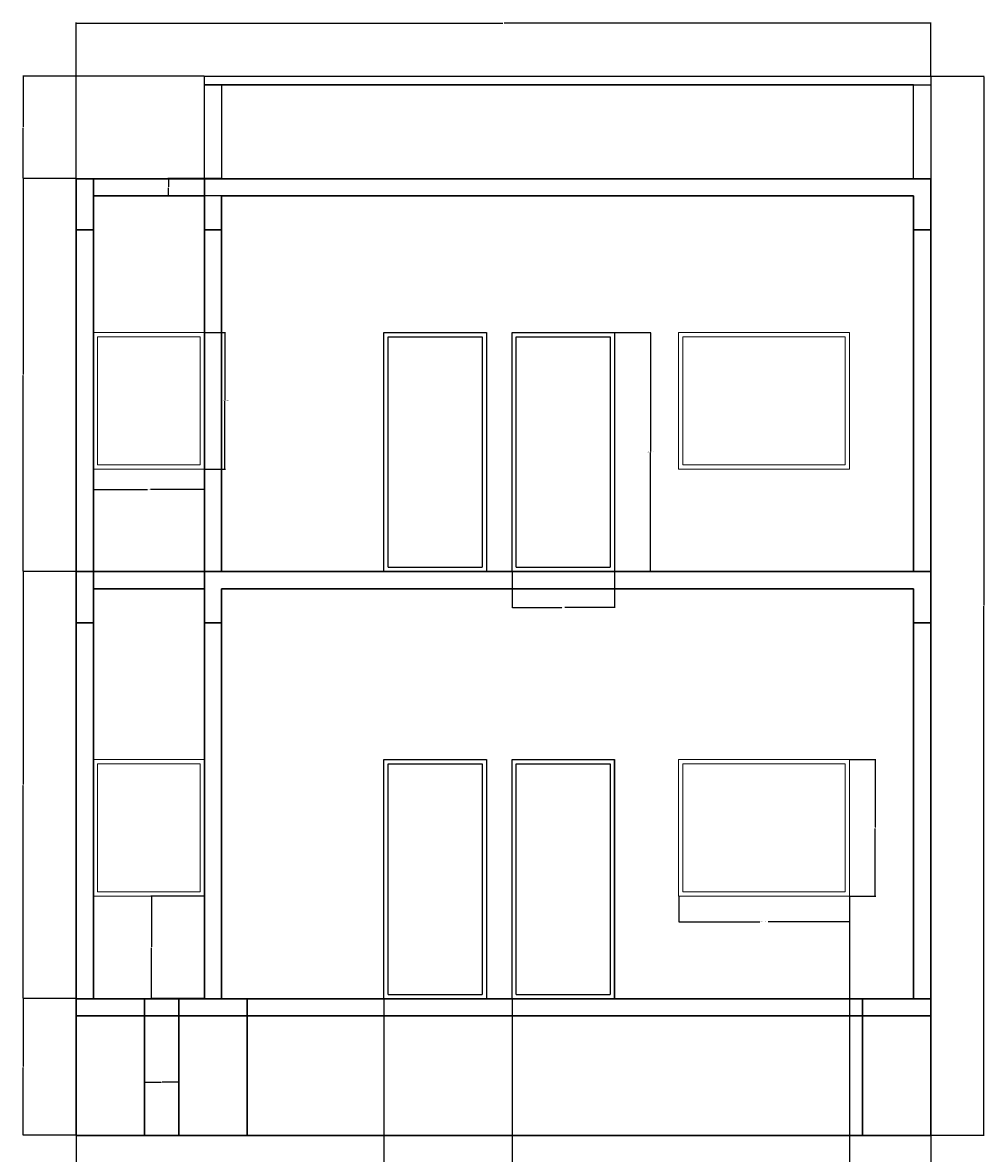
# Model space of a CAD drawing. Units: millimetres. Extents: x 1831 to 2754, y 1517 to 2450.
# Tile 4 of 4: x 2413 to 2751, y 1965 to 2362. Entities that reach past the tile are written whole.
import ezdxf

# ---------------------------------------------------------------- set-up
doc = ezdxf.new("R2010")
doc.units = ezdxf.units.MM
for name, color, linetype, lineweight in [('A-ANNO-DIMS', 2, 'Continuous', 18), ('A-DOOR', 3, 'Continuous', 25), ('A-ELEV-BASE', 7, 'Continuous', 30), ('A-GLAZ', 4, 'Continuous', 18), ('A-ROOF', 7, 'Continuous', 25), ('A-SECT', 7, 'Continuous', 30)]:
    doc.layers.add(name, color=color, linetype=linetype, lineweight=lineweight)
doc.styles.get("Standard").update_dxf_attribs({"font": 'arial.ttf'})
doc.dimstyles.get("Standard").update_dxf_attribs({"dimtxt": 0.18, "dimasz": 0.18, "dimexe": 0.18, "dimexo": 0.0625, "dimgap": 0.09, "dimtad": 0, "dimtih": 1, "dimtoh": 1, "dimdec": 4, "dimzin": 0, "dimdsep": 46, "dimtxsty": 'Standard', "dimcen": 0.09, "dimadec": 0, "dimazin": 0, "dimtfac": 1, "dimtdec": 4, "dimtofl": 0, "dimtmove": 0, "dimatfit": 3, "dimfxl": 1, "dimtolj": 1, "dimtzin": 0, "dimarcsym": 0})

# ---------------------------------------------------------------- blocks, each defined once
blk = doc.blocks.new('DOOR-SECT-FRAMED')
for p, q in [((0, 0), (0, 84)), ((0, 84), (36, 84)), ((36, 84), (36, 0)), ((1.5, 82.5), (34.5, 82.5)), ((1.5, 1.5), (1.5, 82.5)), ((34.5, 82.5), (34.5, 1.5)), ((1.5, 1.5), (34.5, 1.5))]:
    blk.add_line(p, q)
blk = doc.blocks.new('WINDOW-SECT-WIDE')
for p, q in [((0, 48), (60, 48)), ((30, 48), (0, 48)), ((0, 48), (0, 0)), ((60, 48), (30, 48)), ((60, 0), (60, 48)), ((30, 46.5), (1.5, 46.5)), ((1.5, 46.5), (1.5, 1.5)), ((58.5, 46.5), (30, 46.5)), ((58.5, 1.5), (58.5, 46.5)), ((1.5, 1.5), (58.5, 1.5)), ((0, 0), (60, 0))]:
    blk.add_line(p, q)
blk = doc.blocks.new('WINDOW-SECT-NARROW')
for p, q in [((0, 48), (39, 48)), ((39, 48), (39, 0)), ((1.5, 46.5), (37.5, 46.5)), ((1.5, 1.5), (1.5, 46.5)), ((37.5, 46.5), (37.5, 1.5)), ((37.5, 1.5), (1.5, 1.5)), ((39, 0), (0, 0))]:
    blk.add_line(p, q)
blk = doc.blocks.new('*D8')
at = {"layer": 'A-ANNO-DIMS', "color": 0, "lineweight": -2, "transparency": 16777216}
for p, q in [((2620.82, 2253.57), (2633.54, 2253.57)), ((2633.36, 2253.39), (2633.36, 2211.75)), ((2633.36, 2169.75), (2633.36, 2211.38)), ((2620.82, 2169.57), (2633.54, 2169.57))]:
    blk.add_line(p, q, dxfattribs=at)
at = {"layer": 'A-ANNO-DIMS', "color": 0, "transparency": 16777216}
for points in [[(2633.33, 2253.39), (2633.39, 2253.39), (2633.36, 2253.57)], [(2633.33, 2169.75), (2633.39, 2169.75), (2633.36, 2169.57)]]:
    blk.add_solid(points, dxfattribs=at)
at = {"layer": 'Defpoints', "color": 0, "transparency": 16777216}
for p in [(2620.76, 2253.57), (2633.36, 2253.57), (2620.76, 2169.57)]:
    blk.add_point(p, dxfattribs=at)
at = {"layer": 'A-ANNO-DIMS', "color": 0, "transparency": 16777216, "insert": (2633.36, 2211.57), "char_height": 0.18, "attachment_point": 5}
blk.add_mtext('\\A1;FRAMED DOOR 84 TYP.', dxfattribs=at)
blk = doc.blocks.new('*D9')
at = {"layer": 'A-ANNO-DIMS', "color": 0, "lineweight": -2, "transparency": 16777216}
for p, q in [((2584.76, 2169.5), (2584.76, 2156.79)), ((2620.76, 2169.5), (2620.76, 2156.79)), ((2584.94, 2156.97), (2602.23, 2156.97)), ((2620.58, 2156.97), (2603.29, 2156.97))]:
    blk.add_line(p, q, dxfattribs=at)
at = {"layer": 'A-ANNO-DIMS', "color": 0, "transparency": 16777216}
for points in [[(2584.94, 2157), (2584.94, 2156.94), (2584.76, 2156.97)], [(2620.58, 2157), (2620.58, 2156.94), (2620.76, 2156.97)]]:
    blk.add_solid(points, dxfattribs=at)
at = {"layer": 'Defpoints', "color": 0, "transparency": 16777216}
for p in [(2584.76, 2169.57), (2620.76, 2169.57), (2620.76, 2156.97)]:
    blk.add_point(p, dxfattribs=at)
at = {"layer": 'A-ANNO-DIMS', "color": 0, "transparency": 16777216, "insert": (2602.76, 2156.97), "char_height": 0.18, "attachment_point": 5}
blk.add_mtext('\\A1;36 TYP.', dxfattribs=at)
blk = doc.blocks.new('*D10')
at = {"layer": 'A-ANNO-DIMS', "color": 0, "lineweight": -2, "transparency": 16777216}
for p, q in [((2643.26, 2055.5), (2643.26, 2046.39)), ((2703.26, 2055.5), (2703.26, 2046.39)), ((2643.44, 2046.57), (2671.78, 2046.57)), ((2703.08, 2046.57), (2674.74, 2046.57))]:
    blk.add_line(p, q, dxfattribs=at)
at = {"layer": 'A-ANNO-DIMS', "color": 0, "transparency": 16777216}
for points in [[(2643.44, 2046.6), (2643.44, 2046.54), (2643.26, 2046.57)], [(2703.08, 2046.6), (2703.08, 2046.54), (2703.26, 2046.57)]]:
    blk.add_solid(points, dxfattribs=at)
at = {"layer": 'Defpoints', "color": 0, "transparency": 16777216}
for p in [(2643.26, 2055.57), (2703.26, 2055.57), (2703.26, 2046.57)]:
    blk.add_point(p, dxfattribs=at)
at = {"layer": 'A-ANNO-DIMS', "color": 0, "transparency": 16777216, "insert": (2673.26, 2046.57), "char_height": 0.18, "attachment_point": 5}
blk.add_mtext('\\A1;WIDE WINDOW 60 TYP.', dxfattribs=at)
blk = doc.blocks.new('*D11')
at = {"layer": 'A-ANNO-DIMS', "color": 0, "lineweight": -2, "transparency": 16777216}
for p, q in [((2703.32, 2103.57), (2712.44, 2103.57)), ((2712.26, 2103.39), (2712.26, 2079.75)), ((2712.26, 2055.75), (2712.26, 2079.38)), ((2703.32, 2055.57), (2712.44, 2055.57))]:
    blk.add_line(p, q, dxfattribs=at)
at = {"layer": 'A-ANNO-DIMS', "color": 0, "transparency": 16777216}
for points in [[(2712.23, 2103.39), (2712.29, 2103.39), (2712.26, 2103.57)], [(2712.23, 2055.75), (2712.29, 2055.75), (2712.26, 2055.57)]]:
    blk.add_solid(points, dxfattribs=at)
at = {"layer": 'Defpoints', "color": 0, "transparency": 16777216}
for p in [(2703.26, 2103.57), (2712.26, 2103.57), (2703.26, 2055.57)]:
    blk.add_point(p, dxfattribs=at)
at = {"layer": 'A-ANNO-DIMS', "color": 0, "transparency": 16777216, "insert": (2712.26, 2079.57), "char_height": 0.18, "attachment_point": 5}
blk.add_mtext('\\A1;48 TYP.', dxfattribs=at)
blk = doc.blocks.new('*D12')
at = {"layer": 'A-ANNO-DIMS', "color": 0, "lineweight": -2, "transparency": 16777216}
for p, q in [((2476.82, 2253.57), (2484.14, 2253.57)), ((2483.96, 2253.39), (2483.96, 2229.75)), ((2483.96, 2205.75), (2483.96, 2229.38)), ((2476.82, 2205.57), (2484.14, 2205.57))]:
    blk.add_line(p, q, dxfattribs=at)
at = {"layer": 'A-ANNO-DIMS', "color": 0, "transparency": 16777216}
for points in [[(2483.93, 2253.39), (2483.99, 2253.39), (2483.96, 2253.57)], [(2483.93, 2205.75), (2483.99, 2205.75), (2483.96, 2205.57)]]:
    blk.add_solid(points, dxfattribs=at)
at = {"layer": 'Defpoints', "color": 0, "transparency": 16777216}
for p in [(2476.76, 2253.57), (2483.96, 2253.57), (2476.76, 2205.57)]:
    blk.add_point(p, dxfattribs=at)
at = {"layer": 'A-ANNO-DIMS', "color": 0, "transparency": 16777216, "insert": (2483.96, 2229.57), "char_height": 0.18, "attachment_point": 5}
blk.add_mtext('\\A1;NARROW WINDOW 48 TYP.', dxfattribs=at)
blk = doc.blocks.new('*D13')
at = {"layer": 'A-ANNO-DIMS', "color": 0, "lineweight": -2, "transparency": 16777216}
for p, q in [((2437.76, 2205.5), (2437.76, 2198.19)), ((2476.76, 2205.5), (2476.76, 2198.19)), ((2437.94, 2198.37), (2456.73, 2198.37)), ((2476.58, 2198.37), (2457.79, 2198.37))]:
    blk.add_line(p, q, dxfattribs=at)
at = {"layer": 'A-ANNO-DIMS', "color": 0, "transparency": 16777216}
for points in [[(2437.94, 2198.4), (2437.94, 2198.34), (2437.76, 2198.37)], [(2476.58, 2198.4), (2476.58, 2198.34), (2476.76, 2198.37)]]:
    blk.add_solid(points, dxfattribs=at)
at = {"layer": 'Defpoints', "color": 0, "transparency": 16777216}
for p in [(2437.76, 2205.57), (2476.76, 2205.57), (2476.76, 2198.37)]:
    blk.add_point(p, dxfattribs=at)
at = {"layer": 'A-ANNO-DIMS', "color": 0, "transparency": 16777216, "insert": (2457.26, 2198.37), "char_height": 0.18, "attachment_point": 5}
blk.add_mtext('\\A1;39 TYP.', dxfattribs=at)
blk = doc.blocks.new('*D60')
at = {"layer": 'A-ANNO-DIMS', "color": 0, "lineweight": -2, "transparency": 16777216}
for p, q in [((2431.76, 2307.63), (2431.76, 2362.38)), ((2431.94, 2362.2), (2581.47, 2362.2)), ((2731.58, 2362.2), (2582.05, 2362.2)), ((2731.76, 2343.63), (2731.76, 2362.38))]:
    blk.add_line(p, q, dxfattribs=at)
at = {"layer": 'A-ANNO-DIMS', "color": 0, "transparency": 16777216}
for points in [[(2431.94, 2362.23), (2431.94, 2362.17), (2431.76, 2362.2)], [(2731.58, 2362.23), (2731.58, 2362.17), (2731.76, 2362.2)]]:
    blk.add_solid(points, dxfattribs=at)
at = {"layer": 'Defpoints', "color": 0, "transparency": 16777216}
for p in [(2731.76, 2362.2), (2731.76, 2343.57), (2431.76, 2307.57)]:
    blk.add_point(p, dxfattribs=at)
at = {"layer": 'A-ANNO-DIMS', "color": 0, "transparency": 16777216, "insert": (2581.76, 2362.2), "char_height": 0.18, "attachment_point": 5}
blk.add_mtext('\\A1;300', dxfattribs=at)
blk = doc.blocks.new('*D61')
at = {"layer": 'A-ANNO-DIMS', "color": 0, "lineweight": -2, "transparency": 16777216}
for p, q in [((2731.82, 2343.57), (2750.57, 2343.57)), ((2750.39, 2343.39), (2750.39, 2157.75)), ((2750.39, 1971.75), (2750.39, 2157.38)), ((2731.82, 1971.57), (2750.57, 1971.57))]:
    blk.add_line(p, q, dxfattribs=at)
at = {"layer": 'A-ANNO-DIMS', "color": 0, "transparency": 16777216}
for points in [[(2750.36, 2343.39), (2750.42, 2343.39), (2750.39, 2343.57)], [(2750.36, 1971.75), (2750.42, 1971.75), (2750.39, 1971.57)]]:
    blk.add_solid(points, dxfattribs=at)
at = {"layer": 'Defpoints', "color": 0, "transparency": 16777216}
for p in [(2731.76, 2343.57), (2750.39, 2343.57), (2731.76, 1971.57)]:
    blk.add_point(p, dxfattribs=at)
at = {"layer": 'A-ANNO-DIMS', "color": 0, "transparency": 16777216, "insert": (2750.39, 2157.57), "char_height": 0.18, "attachment_point": 5}
blk.add_mtext('\\A1;372', dxfattribs=at)
blk = doc.blocks.new('*D62')
at = {"layer": 'A-ANNO-DIMS', "color": 0, "lineweight": -2, "transparency": 16777216}
for p, q in [((2431.7, 2019.57), (2412.95, 2019.57)), ((2413.13, 2019.39), (2413.13, 1995.75)), ((2413.13, 1971.75), (2413.13, 1995.38)), ((2431.7, 1971.57), (2412.95, 1971.57))]:
    blk.add_line(p, q, dxfattribs=at)
at = {"layer": 'A-ANNO-DIMS', "color": 0, "transparency": 16777216}
for points in [[(2413.1, 2019.39), (2413.16, 2019.39), (2413.13, 2019.57)], [(2413.1, 1971.75), (2413.16, 1971.75), (2413.13, 1971.57)]]:
    blk.add_solid(points, dxfattribs=at)
at = {"layer": 'Defpoints', "color": 0, "transparency": 16777216}
for p in [(2413.13, 2019.57), (2431.76, 2019.57), (2431.76, 1971.57)]:
    blk.add_point(p, dxfattribs=at)
at = {"layer": 'A-ANNO-DIMS', "color": 0, "transparency": 16777216, "insert": (2413.13, 1995.57), "char_height": 0.18, "attachment_point": 5}
blk.add_mtext('\\A1;48', dxfattribs=at)
blk = doc.blocks.new('*D63')
at = {"layer": 'A-ANNO-DIMS', "color": 0, "lineweight": -2, "transparency": 16777216}
for p, q in [((2431.7, 2169.57), (2412.95, 2169.57)), ((2413.13, 2169.39), (2413.13, 2094.75)), ((2413.13, 2019.75), (2413.13, 2094.38)), ((2431.7, 2019.57), (2412.95, 2019.57))]:
    blk.add_line(p, q, dxfattribs=at)
at = {"layer": 'A-ANNO-DIMS', "color": 0, "transparency": 16777216}
for points in [[(2413.1, 2169.39), (2413.16, 2169.39), (2413.13, 2169.57)], [(2413.1, 2019.75), (2413.16, 2019.75), (2413.13, 2019.57)]]:
    blk.add_solid(points, dxfattribs=at)
at = {"layer": 'Defpoints', "color": 0, "transparency": 16777216}
for p in [(2413.13, 2169.57), (2431.76, 2169.57), (2431.76, 2019.57)]:
    blk.add_point(p, dxfattribs=at)
at = {"layer": 'A-ANNO-DIMS', "color": 0, "transparency": 16777216, "insert": (2413.13, 2094.57), "char_height": 0.18, "attachment_point": 5}
blk.add_mtext('\\A1;150', dxfattribs=at)
blk = doc.blocks.new('*D64')
at = {"layer": 'A-ANNO-DIMS', "color": 0, "lineweight": -2, "transparency": 16777216}
for p, q in [((2431.7, 2307.57), (2412.95, 2307.57)), ((2413.13, 2307.39), (2413.13, 2238.75)), ((2413.13, 2169.75), (2413.13, 2238.38)), ((2431.7, 2169.57), (2412.95, 2169.57))]:
    blk.add_line(p, q, dxfattribs=at)
at = {"layer": 'A-ANNO-DIMS', "color": 0, "transparency": 16777216}
for points in [[(2413.1, 2307.39), (2413.16, 2307.39), (2413.13, 2307.57)], [(2413.1, 2169.75), (2413.16, 2169.75), (2413.13, 2169.57)]]:
    blk.add_solid(points, dxfattribs=at)
at = {"layer": 'Defpoints', "color": 0, "transparency": 16777216}
for p in [(2413.13, 2307.57), (2431.76, 2307.57), (2431.76, 2169.57)]:
    blk.add_point(p, dxfattribs=at)
at = {"layer": 'A-ANNO-DIMS', "color": 0, "transparency": 16777216, "insert": (2413.13, 2238.57), "char_height": 0.18, "attachment_point": 5}
blk.add_mtext('\\A1;138', dxfattribs=at)
blk = doc.blocks.new('*D65')
at = {"layer": 'A-ANNO-DIMS', "color": 0, "lineweight": -2, "transparency": 16777216}
for p, q in [((2476.7, 2343.57), (2412.95, 2343.57)), ((2413.13, 2343.39), (2413.13, 2325.75)), ((2413.13, 2307.75), (2413.13, 2325.38)), ((2431.7, 2307.57), (2412.95, 2307.57))]:
    blk.add_line(p, q, dxfattribs=at)
at = {"layer": 'A-ANNO-DIMS', "color": 0, "transparency": 16777216}
for points in [[(2413.1, 2343.39), (2413.16, 2343.39), (2413.13, 2343.57)], [(2413.1, 2307.75), (2413.16, 2307.75), (2413.13, 2307.57)]]:
    blk.add_solid(points, dxfattribs=at)
at = {"layer": 'Defpoints', "color": 0, "transparency": 16777216}
for p in [(2413.13, 2343.57), (2476.76, 2343.57), (2431.76, 2307.57)]:
    blk.add_point(p, dxfattribs=at)
at = {"layer": 'A-ANNO-DIMS', "color": 0, "transparency": 16777216, "insert": (2413.13, 2325.57), "char_height": 0.18, "attachment_point": 5}
blk.add_mtext('\\A1;36', dxfattribs=at)
blk = doc.blocks.new('*D66')
at = {"layer": 'A-ANNO-DIMS', "color": 0, "lineweight": -2, "transparency": 16777216}
for p, q in [((2476.7, 2055.57), (2457.95, 2055.57)), ((2458.13, 2055.39), (2458.13, 2037.75)), ((2458.13, 2019.75), (2458.13, 2037.38)), ((2476.7, 2019.57), (2457.95, 2019.57))]:
    blk.add_line(p, q, dxfattribs=at)
at = {"layer": 'A-ANNO-DIMS', "color": 0, "transparency": 16777216}
for points in [[(2458.1, 2055.39), (2458.16, 2055.39), (2458.13, 2055.57)], [(2458.1, 2019.75), (2458.16, 2019.75), (2458.13, 2019.57)]]:
    blk.add_solid(points, dxfattribs=at)
at = {"layer": 'Defpoints', "color": 0, "transparency": 16777216}
for p in [(2458.13, 2055.57), (2476.76, 2055.57), (2476.76, 2019.57)]:
    blk.add_point(p, dxfattribs=at)
at = {"layer": 'A-ANNO-DIMS', "color": 0, "transparency": 16777216, "insert": (2458.13, 2037.57), "char_height": 0.18, "attachment_point": 5}
blk.add_mtext('\\A1;36', dxfattribs=at)
blk = doc.blocks.new('*D67')
at = {"layer": 'A-ANNO-DIMS', "color": 0, "lineweight": -2, "transparency": 16777216}
for p, q in [((2431.76, 2019.5), (2431.76, 1952.75)), ((2539.76, 2019.5), (2539.76, 1952.75)), ((2431.94, 1952.93), (2485.48, 1952.93)), ((2539.58, 1952.93), (2486.04, 1952.93))]:
    blk.add_line(p, q, dxfattribs=at)
at = {"layer": 'A-ANNO-DIMS', "color": 0, "transparency": 16777216}
for points in [[(2431.94, 1952.96), (2431.94, 1952.9), (2431.76, 1952.93)], [(2539.58, 1952.96), (2539.58, 1952.9), (2539.76, 1952.93)]]:
    blk.add_solid(points, dxfattribs=at)
at = {"layer": 'Defpoints', "color": 0, "transparency": 16777216}
for p in [(2431.76, 2019.57), (2539.76, 2019.57), (2539.76, 1952.93)]:
    blk.add_point(p, dxfattribs=at)
at = {"layer": 'A-ANNO-DIMS', "color": 0, "transparency": 16777216, "insert": (2485.76, 1952.93), "char_height": 0.18, "attachment_point": 5}
blk.add_mtext('\\A1;108', dxfattribs=at)
blk = doc.blocks.new('*D68')
at = {"layer": 'A-ANNO-DIMS', "color": 0, "lineweight": -2, "transparency": 16777216}
for p, q in [((2539.76, 2019.5), (2539.76, 1952.75)), ((2584.76, 2019.5), (2584.76, 1952.75)), ((2539.94, 1952.93), (2562.04, 1952.93)), ((2584.58, 1952.93), (2562.48, 1952.93))]:
    blk.add_line(p, q, dxfattribs=at)
at = {"layer": 'A-ANNO-DIMS', "color": 0, "transparency": 16777216}
for points in [[(2539.94, 1952.96), (2539.94, 1952.9), (2539.76, 1952.93)], [(2584.58, 1952.96), (2584.58, 1952.9), (2584.76, 1952.93)]]:
    blk.add_solid(points, dxfattribs=at)
at = {"layer": 'Defpoints', "color": 0, "transparency": 16777216}
for p in [(2539.76, 2019.57), (2584.76, 2019.57), (2584.76, 1952.93)]:
    blk.add_point(p, dxfattribs=at)
at = {"layer": 'A-ANNO-DIMS', "color": 0, "transparency": 16777216, "insert": (2562.26, 1952.93), "char_height": 0.18, "attachment_point": 5}
blk.add_mtext('\\A1;45', dxfattribs=at)
blk = doc.blocks.new('*D69')
at = {"layer": 'A-ANNO-DIMS', "color": 0, "lineweight": -2, "transparency": 16777216}
for p, q in [((2703.26, 2055.5), (2703.26, 1952.75)), ((2731.76, 2019.5), (2731.76, 1952.75)), ((2703.44, 1952.93), (2717.18, 1952.93)), ((2731.58, 1952.93), (2717.83, 1952.93))]:
    blk.add_line(p, q, dxfattribs=at)
at = {"layer": 'A-ANNO-DIMS', "color": 0, "transparency": 16777216}
for points in [[(2703.44, 1952.96), (2703.44, 1952.9), (2703.26, 1952.93)], [(2731.58, 1952.96), (2731.58, 1952.9), (2731.76, 1952.93)]]:
    blk.add_solid(points, dxfattribs=at)
at = {"layer": 'Defpoints', "color": 0, "transparency": 16777216}
for p in [(2703.26, 2055.57), (2731.76, 2019.57), (2731.76, 1952.93)]:
    blk.add_point(p, dxfattribs=at)
at = {"layer": 'A-ANNO-DIMS', "color": 0, "transparency": 16777216, "insert": (2717.51, 1952.93), "char_height": 0.18, "attachment_point": 5}
blk.add_mtext('\\A1;28.5', dxfattribs=at)
blk = doc.blocks.new('*D70')
at = {"layer": 'A-ANNO-DIMS', "color": 0, "lineweight": -2, "transparency": 16777216}
for p, q in [((2482.7, 2307.57), (2463.95, 2307.57)), ((2464.13, 2307.39), (2464.13, 2304.75)), ((2464.13, 2301.75), (2464.13, 2304.38)), ((2482.7, 2301.57), (2463.95, 2301.57))]:
    blk.add_line(p, q, dxfattribs=at)
at = {"layer": 'A-ANNO-DIMS', "color": 0, "transparency": 16777216}
for points in [[(2464.1, 2307.39), (2464.16, 2307.39), (2464.13, 2307.57)], [(2464.1, 2301.75), (2464.16, 2301.75), (2464.13, 2301.57)]]:
    blk.add_solid(points, dxfattribs=at)
at = {"layer": 'Defpoints', "color": 0, "transparency": 16777216}
for p in [(2464.13, 2307.57), (2482.76, 2307.57), (2482.76, 2301.57)]:
    blk.add_point(p, dxfattribs=at)
at = {"layer": 'A-ANNO-DIMS', "color": 0, "transparency": 16777216, "insert": (2464.13, 2304.57), "char_height": 0.18, "attachment_point": 5}
blk.add_mtext('\\A1;6', dxfattribs=at)
blk = doc.blocks.new('*D71')
at = {"layer": 'A-ANNO-DIMS', "color": 0, "lineweight": -2, "transparency": 16777216}
for p, q in [((2455.76, 1971.63), (2455.76, 1990.38)), ((2455.94, 1990.2), (2461.55, 1990.2)), ((2467.58, 1990.2), (2461.97, 1990.2)), ((2467.76, 1971.63), (2467.76, 1990.38))]:
    blk.add_line(p, q, dxfattribs=at)
at = {"layer": 'A-ANNO-DIMS', "color": 0, "transparency": 16777216}
for points in [[(2455.94, 1990.23), (2455.94, 1990.17), (2455.76, 1990.2)], [(2467.58, 1990.23), (2467.58, 1990.17), (2467.76, 1990.2)]]:
    blk.add_solid(points, dxfattribs=at)
at = {"layer": 'Defpoints', "color": 0, "transparency": 16777216}
for p in [(2467.76, 1990.2), (2455.76, 1971.57), (2467.76, 1971.57)]:
    blk.add_point(p, dxfattribs=at)
at = {"layer": 'A-ANNO-DIMS', "color": 0, "transparency": 16777216, "insert": (2461.76, 1990.2), "char_height": 0.18, "attachment_point": 5}
blk.add_mtext('\\A1;12', dxfattribs=at)

msp = doc.modelspace()

# ---------------------------------------------------------------- linework, layer by layer
at = {"layer": 'A-DOOR'}
msp.add_line((2620.758, 2019.566), (2620.758, 2103.566), dxfattribs=at)
at = {"layer": 'A-ELEV-BASE'}
for p, q in [((2431.758, 1971.566), (2431.758, 2019.566)), ((2431.758, 2019.566), (2455.758, 2019.566)), ((2431.758, 2019.566), (2431.758, 2013.566)), ((2455.758, 2019.566), (2455.758, 1971.566)), ((2467.758, 1971.566), (2467.758, 2019.566)), ((2467.758, 2019.566), (2491.758, 2019.566)), ((2491.758, 2019.566), (2491.758, 1971.566)), ((2731.758, 2019.566), (2707.758, 2019.566)), ((2707.758, 2019.566), (2707.758, 1971.566)), ((2731.758, 1971.566), (2731.758, 2019.566)), ((2431.758, 2013.566), (2731.758, 2013.566)), ((2455.758, 1971.566), (2431.758, 1971.566)), ((2431.758, 1971.566), (2455.758, 1971.566)), ((2467.758, 1971.566), (2431.758, 1971.566)), ((2431.758, 1971.566), (2731.758, 1971.566)), ((2455.758, 1971.566), (2467.758, 1971.566)), ((2491.758, 1971.566), (2467.758, 1971.566))]:
    msp.add_line(p, q, dxfattribs=at)
at = {"layer": 'A-ROOF'}
for p, q in [((2476.758, 2307.566), (2476.758, 2343.566)), ((2476.758, 2343.566), (2731.758, 2343.566)), ((2731.758, 2343.566), (2731.758, 2307.566)), ((2482.758, 2340.566), (2476.758, 2340.566)), ((2476.758, 2340.566), (2731.758, 2340.566)), ((2725.758, 2340.566), (2482.758, 2340.566)), ((2482.758, 2340.566), (2482.758, 2307.566)), ((2725.758, 2307.566), (2725.758, 2340.566))]:
    msp.add_line(p, q, dxfattribs=at)
at = {"layer": 'A-SECT'}
for p, q in [((2431.758, 2169.566), (2431.758, 2307.566)), ((2431.758, 2301.566), (2431.758, 2307.566)), ((2431.758, 2307.566), (2731.758, 2307.566)), ((2431.758, 2307.566), (2431.758, 2289.566)), ((2437.758, 2301.566), (2437.758, 2307.566)), ((2476.758, 2169.566), (2476.758, 2307.566)), ((2476.758, 2307.566), (2482.758, 2307.566)), ((2731.758, 2307.566), (2725.758, 2307.566)), ((2731.758, 2307.566), (2731.758, 2169.566)), ((2437.758, 2169.566), (2437.758, 2301.566)), ((2437.758, 2301.566), (2476.758, 2301.566)), ((2482.758, 2169.566), (2482.758, 2301.566)), ((2482.758, 2301.566), (2725.758, 2301.566)), ((2482.758, 2301.566), (2482.758, 2289.566)), ((2725.758, 2301.566), (2725.758, 2169.566)), ((2725.758, 2301.566), (2725.758, 2289.566)), ((2431.758, 2289.566), (2437.758, 2289.566)), ((2482.758, 2289.566), (2476.758, 2289.566)), ((2725.758, 2289.566), (2731.758, 2289.566)), ((2437.758, 2169.566), (2437.758, 2253.566)), ((2431.758, 2163.566), (2431.758, 2169.566)), ((2431.758, 2169.566), (2731.758, 2169.566)), ((2431.758, 2169.566), (2431.758, 2151.566)), ((2437.758, 2151.566), (2437.758, 2169.566)), ((2437.758, 2169.566), (2437.758, 2169.566)), ((2482.758, 2169.566), (2476.758, 2169.566)), ((2476.758, 2169.566), (2476.758, 2151.566)), ((2575.758, 2169.566), (2584.758, 2169.566)), ((2731.758, 2169.566), (2725.758, 2169.566)), ((2731.758, 2169.566), (2731.758, 2163.566)), ((2731.758, 2169.566), (2731.758, 2151.566)), ((2431.758, 2019.566), (2431.758, 2163.566)), ((2437.758, 2019.566), (2437.758, 2163.566)), ((2437.758, 2163.566), (2476.758, 2163.566)), ((2476.758, 2019.566), (2476.758, 2163.566)), ((2482.758, 2019.566), (2482.758, 2163.566)), ((2482.758, 2163.566), (2725.758, 2163.566)), ((2725.758, 2163.566), (2725.758, 2019.566)), ((2731.758, 2163.566), (2731.758, 2019.566)), ((2431.758, 2151.566), (2437.758, 2151.566)), ((2476.758, 2151.566), (2482.758, 2151.566)), ((2731.758, 2151.566), (2725.758, 2151.566)), ((2437.758, 2019.566), (2437.758, 2103.566)), ((2731.758, 2019.566), (2431.758, 2019.566)), ((2431.758, 2019.566), (2437.758, 2019.566)), ((2491.758, 2019.566), (2479.758, 2019.566)), ((2482.758, 2019.566), (2530.758, 2019.566)), ((2530.758, 2019.566), (2536.758, 2019.566)), ((2536.758, 2019.566), (2539.758, 2019.566)), ((2575.758, 2019.566), (2584.758, 2019.566))]:
    msp.add_line(p, q, dxfattribs=at)

# ---------------------------------------------------------------- block references
at = {"layer": 'A-DOOR'}
for p in [(2539.758, 2169.566), (2584.758, 2169.566), (2539.758, 2019.566), (2584.758, 2019.566)]:
    msp.add_blockref('DOOR-SECT-FRAMED', p, dxfattribs=at)
at = {"layer": 'A-GLAZ'}
for name, p in [('WINDOW-SECT-NARROW', (2437.758, 2205.566)), ('WINDOW-SECT-WIDE', (2643.258, 2205.566)), ('WINDOW-SECT-NARROW', (2437.758, 2055.566)), ('WINDOW-SECT-WIDE', (2643.258, 2055.566))]:
    msp.add_blockref(name, p, dxfattribs=at)

# ---------------------------------------------------------------- dimensions: what is measured, and where the dimension line sits
at = {"layer": 'A-ANNO-DIMS'}
for base, p1, p2, override, picture, middle in [((2731.758, 2362.198), (2431.758, 2307.566), (2731.758, 2343.566), {"dimdec": 0, "dimlfac": 1, "dimrnd": 0, "dimzin": 0, "dimdsep": 46, "dimlunit": 2}, '*D60', (2581.758, 2362.198)), ((2731.758, 1952.933), (2703.258, 2055.566), (2731.758, 2019.566), {"dimdec": 1, "dimlfac": 1, "dimrnd": 0, "dimzin": 0, "dimdsep": 46, "dimlunit": 2}, '*D69', (2717.508, 1952.933)), ((2539.758, 1952.933), (2431.758, 2019.566), (2539.758, 2019.566), {"dimdec": 0, "dimlfac": 1, "dimrnd": 0, "dimzin": 0, "dimdsep": 46, "dimlunit": 2}, '*D67', (2485.758, 1952.933)), ((2584.758, 1952.933), (2539.758, 2019.566), (2584.758, 2019.566), {"dimdec": 0, "dimlfac": 1, "dimrnd": 0, "dimzin": 0, "dimdsep": 46, "dimlunit": 2}, '*D68', (2562.258, 1952.933)), ((2467.758, 1990.198), (2455.758, 1971.566), (2467.758, 1971.566), {"dimdec": 0, "dimlfac": 1, "dimrnd": 0, "dimzin": 0, "dimdsep": 46, "dimlunit": 2}, '*D71', (2461.758, 1990.198))]:
    dim = msp.add_linear_dim(base=base, p1=p1, p2=p2, dimstyle='Standard', override=override, dxfattribs=at)
    dim.commit()
    dim.dimension.update_dxf_attribs({"geometry": picture, "text_midpoint": middle})
for base, p1, p2, picture, middle in [((2413.126, 2343.566), (2431.758, 2307.566), (2476.758, 2343.566), '*D65', (2413.126, 2325.566)), ((2750.391, 2343.566), (2731.758, 1971.566), (2731.758, 2343.566), '*D61', (2750.391, 2157.566)), ((2413.126, 2307.566), (2431.758, 2169.566), (2431.758, 2307.566), '*D64', (2413.126, 2238.566)), ((2464.126, 2307.566), (2482.758, 2301.566), (2482.758, 2307.566), '*D70', (2464.126, 2304.566)), ((2413.126, 2169.566), (2431.758, 2019.566), (2431.758, 2169.566), '*D63', (2413.126, 2094.566)), ((2458.126, 2055.566), (2476.758, 2019.566), (2476.758, 2055.566), '*D66', (2458.126, 2037.566)), ((2413.126, 2019.566), (2431.758, 1971.566), (2431.758, 2019.566), '*D62', (2413.126, 1995.566))]:
    dim = msp.add_linear_dim(base=base, p1=p1, p2=p2, angle=90, dimstyle='Standard', override={"dimdec": 0, "dimlfac": 1, "dimrnd": 0, "dimzin": 0, "dimdsep": 46, "dimlunit": 2}, dxfattribs=at)
    dim.commit()
    dim.dimension.update_dxf_attribs({"geometry": picture, "text_midpoint": middle})
for base, p1, p2, text, picture, middle in [((2483.958, 2253.566), (2476.758, 2205.566), (2476.758, 2253.566), 'NARROW WINDOW <> TYP.', '*D12', (2483.958, 2229.566)), ((2633.358, 2253.566), (2620.758, 2169.566), (2620.758, 2253.566), 'FRAMED DOOR <> TYP.', '*D8', (2633.358, 2211.566)), ((2712.258, 2103.566), (2703.258, 2055.566), (2703.258, 2103.566), '<> TYP.', '*D11', (2712.258, 2079.566))]:
    dim = msp.add_linear_dim(base=base, p1=p1, p2=p2, angle=90, text=text, dimstyle='Standard', override={"dimdec": 0, "dimlfac": 1, "dimrnd": 0, "dimzin": 0, "dimdsep": 46, "dimlunit": 2}, dxfattribs=at)
    dim.commit()
    dim.dimension.update_dxf_attribs({"geometry": picture, "text_midpoint": middle})
for base, p1, p2, text, picture, middle in [((2476.758, 2198.366), (2437.758, 2205.566), (2476.758, 2205.566), '<> TYP.', '*D13', (2457.258, 2198.366)), ((2620.758, 2156.966), (2584.758, 2169.566), (2620.758, 2169.566), '<> TYP.', '*D9', (2602.758, 2156.966)), ((2703.258, 2046.566), (2643.258, 2055.566), (2703.258, 2055.566), 'WIDE WINDOW <> TYP.', '*D10', (2673.258, 2046.566))]:
    dim = msp.add_linear_dim(base=base, p1=p1, p2=p2, text=text, dimstyle='Standard', override={"dimdec": 0, "dimlfac": 1, "dimrnd": 0, "dimzin": 0, "dimdsep": 46, "dimlunit": 2}, dxfattribs=at)
    dim.commit()
    dim.dimension.update_dxf_attribs({"geometry": picture, "text_midpoint": middle})

doc.saveas('drawing.dxf')
